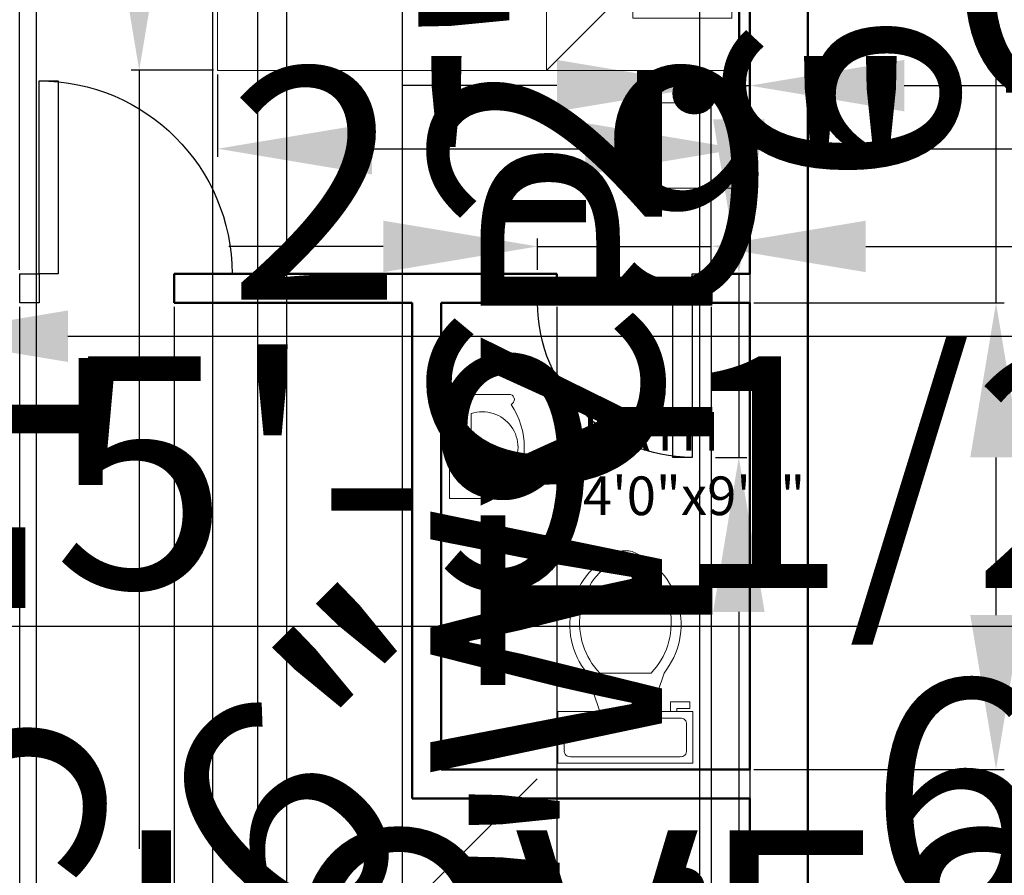
# Model space of a CAD drawing. Units: inches. Extents: x 1102 to 2414, y 295 to 1561.
# Tile 7 of 11: x 1695 to 1848, y 894 to 1027. Entities that reach past the tile are written whole.
import ezdxf

# ---------------------------------------------------------------- set-up
doc = ezdxf.new("R2010")
doc.units = ezdxf.units.IN
for name, color, linetype, lineweight in [('A-ANNO-DIMS', 2, 'Continuous', 18), ('A-AREA-IDEN', 7, 'Continuous', 25), ('A-DOOR', 4, 'Continuous', 25), ('A-FLOR-FIXT', 9, 'Continuous', 18), ('A-FURN', 8, 'Continuous', 18), ('A-WALL', 7, 'Continuous', 50)]:
    doc.layers.add(name, color=color, linetype=linetype, lineweight=lineweight)
doc.styles.get("Standard").update_dxf_attribs({"font": 'arial.ttf'})
doc.dimstyles.new('ISO-25', dxfattribs={"dimtxt": 36, "dimasz": 24, "dimexe": 1.25, "dimexo": 0.625, "dimtad": 1, "dimlunit": 4, "dimtxsty": 'Standard', "dimcen": 2.5, "dimadec": 0, "dimazin": 0, "dimtfac": 1, "dimtmove": 0, "dimatfit": 3, "dimfxl": 1, "dimarcsym": 0})

# ---------------------------------------------------------------- blocks, each defined once
blk = doc.blocks.new('*D3')
at = {"layer": 'A-ANNO-DIMS', "color": 0, "lineweight": -2, "transparency": 16777216}
for p, q in [((1818.17, 1116.76), (1895.42, 1116.76)), ((1894.17, 1092.76), (1894.17, 660.76)), ((1818.17, 636.76), (1895.42, 636.76))]:
    blk.add_line(p, q, dxfattribs=at)
at = {"layer": 'A-ANNO-DIMS', "color": 0, "transparency": 16777216}
for points in [[(1890.17, 1092.76), (1898.17, 1092.76), (1894.17, 1116.76)], [(1890.17, 660.76), (1898.17, 660.76), (1894.17, 636.76)]]:
    blk.add_solid(points, dxfattribs=at)
at = {"layer": 'Defpoints', "color": 0, "transparency": 16777216}
for p in [(1817.54, 1116.76), (1817.54, 636.76), (1894.17, 636.76)]:
    blk.add_point(p, dxfattribs=at)
at = {"layer": 'A-ANNO-DIMS', "color": 0, "transparency": 16777216, "insert": (1875.16, 876.76), "char_height": 36, "attachment_point": 5, "rotation": 90}
blk.add_mtext("40'", dxfattribs=at)
blk = doc.blocks.new('Toilet - top')
for p, q in [((9.5, -6), (9.5, -2)), ((-10, -8.5), (-8, -8.5)), ((-10, -9.5), (-10, -8.5)), ((-8, -8.5), (-8, -8)), ((-7, -8), (-7, -9.5)), ((-4, -8), (-6, -14)), ((4, -8), (6, -14)), ((-7, -9.5), (-10, -9.5)), ((4, -14), (-4, -14))]:
    blk.add_line(p, q)
blk.add_lwpolyline([(10.5, -8), (10.5, 0), (-10.5, 0), (-10.5, -8)], close=True)
for points in [[(8.5, -1), (-8.5, -1)], [(-9.5, -2), (-9.5, -6)], [(-8.5, -7), (8.5, -7)]]:
    blk.add_lwpolyline(points)
for centre, radius, start, end in [((-8.62, -1.88), 0.884, 81.8699, 188.1301), ((8.62, -1.88), 0.884, 351.8699, 98.1301), ((-8.62, -6.12), 0.884, 171.8699, 278.1301), ((8.62, -6.12), 0.884, 261.8699, 8.1301), ((3.52, -21.58), 12.17, 141.4691, 247.9714), ((4.2, -21.82), 11.33, 136.3677, 238.9468), ((-3.52, -21.58), 12.17, 292.0284, 38.5307), ((-4.2, -21.82), 11.33, 301.053, 43.6321), ((0, -27.88), 4, 245.7318, 294.2682), ((0, -29), 4, 254.8605, 285.1395)]:
    blk.add_arc(centre, radius, start, end)
blk = doc.blocks.new('Bed - Queen')
for p, q in [((0, -80.00003), (0, 0)), ((0, 0), (59.99999, 0)), ((59.99999, 0), (59.99999, -80.00003)), ((7.99999, -1.2), (28.79998, -1.2)), ((7.99999, -14.4), (7.99999, -1.2)), ((28.79998, -1.2), (28.79998, -14.4)), ((31.19999, -1.2), (51.99999, -1.2)), ((31.19999, -14.4), (31.19999, -1.2)), ((51.99999, -1.2), (51.99999, -16.4)), ((0, -14.4), (44.8, -14.4)), ((59.99999, -29.6), (44.8, -14.4)), ((44.8, -14.4), (44.8, -29.6)), ((51.99999, -16.4), (46.79936, -16.4)), ((44.8, -16.8), (0, -16.8)), ((44.8, -29.6), (59.99999, -29.6)), ((59.99999, -80.00003), (0, -80.00003))]:
    blk.add_line(p, q)
blk = doc.blocks.new('roomdoor')
for points in [[(1837.54, 1413.02), (1840.54, 1413.02), (1840.54, 1443.02), (1837.54, 1443.02)], [(1840.54, 1408.52), (1843.54, 1408.52), (1843.54, 1413.02), (1840.54, 1413.02)]]:
    blk.add_lwpolyline(points, close=True)
blk.add_arc((1840.54, 1413.02), 30, 90, 180)
blk = doc.blocks.new('utilitydoor')
for points in [[(1891.43, 1413.69), (1894.43, 1413.69), (1894.43, 1437.69), (1891.43, 1437.69)], [(1894.43, 1409.19), (1897.43, 1409.19), (1897.43, 1413.69), (1894.43, 1413.69)]]:
    blk.add_lwpolyline(points, close=True)
blk.add_arc((1894.43, 1413.69), 24, 90, 180)
blk = doc.blocks.new('TABLE-BEDSIDE')
for p, q in [((16.99, 13.29), (0, 13.29)), ((0, 13.29), (0, 0)), ((2.56, 0), (2.56, 13.29)), ((16.99, 0), (16.99, 13.29)), ((0, 0), (16.99, 0))]:
    blk.add_line(p, q)
blk = doc.blocks.new('*D18')
at = {"layer": 'A-ANNO-DIMS', "color": 0, "lineweight": -2, "transparency": 16777216}
for p, q in [((1646.02, 927.81), (1646.02, 951.81)), ((1643.89, 903.81), (1647.27, 903.81)), ((1646.02, 903.81), (1646.02, 894.61)), ((1643.89, 894.6), (1647.27, 894.61)), ((1646.03, 870.61), (1646.05, 625.92))]:
    blk.add_line(p, q, dxfattribs=at)
at = {"layer": 'A-ANNO-DIMS', "color": 0, "transparency": 16777216}
for points in [[(1650.02, 927.81), (1642.02, 927.81), (1646.02, 903.81)], [(1650.03, 870.61), (1642.03, 870.6), (1646.02, 894.61)]]:
    blk.add_solid(points, dxfattribs=at)
at = {"layer": 'Defpoints', "color": 0, "transparency": 16777216}
for p in [(1643.27, 903.81), (1643.27, 894.6), (1646.02, 894.61)]:
    blk.add_point(p, dxfattribs=at)
at = {"layer": 'A-ANNO-DIMS', "color": 0, "transparency": 16777216, "insert": (1665.05, 736.26), "char_height": 36, "attachment_point": 5, "rotation": 270.0057}
blk.add_mtext('0\'-9" TYP.', dxfattribs=at)
blk = doc.blocks.new('*D20')
at = {"layer": 'A-ANNO-DIMS', "color": 0, "lineweight": -2, "transparency": 16777216}
for p, q in [((1808.58, 695.77), (1808.58, 1020.95)), ((1806.65, 671.77), (1809.83, 671.77)), ((1808.58, 658.48), (1808.58, 671.77)), ((1806.65, 658.48), (1809.83, 658.48)), ((1808.58, 634.48), (1808.58, 610.48))]:
    blk.add_line(p, q, dxfattribs=at)
at = {"layer": 'A-ANNO-DIMS', "color": 0, "transparency": 16777216}
for points in [[(1804.58, 695.77), (1812.58, 695.77), (1808.58, 671.77)], [(1804.58, 634.48), (1812.58, 634.48), (1808.58, 658.48)]]:
    blk.add_solid(points, dxfattribs=at)
at = {"layer": 'Defpoints', "color": 0, "transparency": 16777216}
for p in [(1806.03, 671.77), (1808.58, 671.77), (1806.03, 658.48)]:
    blk.add_point(p, dxfattribs=at)
at = {"layer": 'A-ANNO-DIMS', "color": 0, "transparency": 16777216, "insert": (1789.34, 870.36), "char_height": 36, "attachment_point": 5, "rotation": 90}
blk.add_mtext('1\'-1 1/2" TYP.', dxfattribs=at)
blk = doc.blocks.new('*D23')
at = {"layer": 'A-ANNO-DIMS', "color": 0, "lineweight": -2, "transparency": 16777216}
for p, q in [((1725.8, 1018.76), (1725.8, 1005.96)), ((1806.97, 1018.76), (1806.97, 1005.96)), ((1749.8, 1007.21), (1782.97, 1007.21)), ((1806.97, 1007.21), (2238.05, 1007.21))]:
    blk.add_line(p, q, dxfattribs=at)
at = {"layer": 'A-ANNO-DIMS', "color": 0, "transparency": 16777216}
for points in [[(1749.8, 1011.21), (1749.8, 1003.21), (1725.8, 1007.21)], [(1782.97, 1011.21), (1782.97, 1003.21), (1806.97, 1007.21)]]:
    blk.add_solid(points, dxfattribs=at)
at = {"layer": 'Defpoints', "color": 0, "transparency": 16777216}
for p in [(1725.8, 1019.39), (1806.97, 1019.39), (1806.97, 1007.21)]:
    blk.add_point(p, dxfattribs=at)
at = {"layer": 'A-ANNO-DIMS', "color": 0, "transparency": 16777216, "insert": (2034.51, 1027.55), "char_height": 36, "attachment_point": 5}
blk.add_mtext('QUEEN BED 6\'-9"', dxfattribs=at)
blk = doc.blocks.new('*D24')
at = {"layer": 'A-ANNO-DIMS', "color": 0, "lineweight": -2, "transparency": 16777216}
for p, q in [((1725.17, 1080.27), (1712.37, 1080.27)), ((1713.62, 1056.27), (1713.62, 1043.39)), ((1725.17, 1019.39), (1712.37, 1019.39)), ((1713.62, 1019.39), (1713.62, 898.44))]:
    blk.add_line(p, q, dxfattribs=at)
at = {"layer": 'A-ANNO-DIMS', "color": 0, "transparency": 16777216}
for points in [[(1709.62, 1056.27), (1717.62, 1056.27), (1713.62, 1080.27)], [(1709.62, 1043.39), (1717.62, 1043.39), (1713.62, 1019.39)]]:
    blk.add_solid(points, dxfattribs=at)
at = {"layer": 'Defpoints', "color": 0, "transparency": 16777216}
for p in [(1725.8, 1080.27), (1713.62, 1019.39), (1725.8, 1019.39)]:
    blk.add_point(p, dxfattribs=at)
at = {"layer": 'A-ANNO-DIMS', "color": 0, "transparency": 16777216, "insert": (1694.62, 946.91), "char_height": 36, "attachment_point": 5, "rotation": 90}
blk.add_mtext('5\'-1"', dxfattribs=at)
blk = doc.blocks.new('*D25')
at = {"layer": 'A-ANNO-DIMS', "color": 0, "lineweight": -2, "transparency": 16777216}
for p, q in [((1800.76, 877.69), (1800.76, 1221.61)), ((1796.43, 853.69), (1802.01, 853.69)), ((1800.76, 820.65), (1800.76, 853.69)), ((1796.43, 820.65), (1802.01, 820.65)), ((1800.76, 796.65), (1800.76, 772.65))]:
    blk.add_line(p, q, dxfattribs=at)
at = {"layer": 'A-ANNO-DIMS', "color": 0, "transparency": 16777216}
for points in [[(1796.76, 877.69), (1804.76, 877.69), (1800.76, 853.69)], [(1796.76, 796.65), (1804.76, 796.65), (1800.76, 820.65)]]:
    blk.add_solid(points, dxfattribs=at)
at = {"layer": 'Defpoints', "color": 0, "transparency": 16777216}
for p in [(1795.81, 853.69), (1800.76, 853.69), (1795.81, 820.65)]:
    blk.add_point(p, dxfattribs=at)
at = {"layer": 'A-ANNO-DIMS', "color": 0, "transparency": 16777216, "insert": (1781.53, 1061.65), "char_height": 36, "attachment_point": 5, "rotation": 90}
blk.add_mtext('WC 2\'-9" TYP.', dxfattribs=at)
blk = doc.blocks.new('*D27')
at = {"layer": 'A-ANNO-DIMS', "color": 0, "lineweight": -2, "transparency": 16777216}
for p, q in [((1683.72, 1041.76), (1683.72, 1561.36)), ((1679.17, 1017.76), (1684.97, 1017.76)), ((1683.72, 983.26), (1683.72, 1017.76)), ((1679.17, 983.26), (1684.97, 983.26)), ((1683.72, 959.26), (1683.72, 935.26))]:
    blk.add_line(p, q, dxfattribs=at)
at = {"layer": 'A-ANNO-DIMS', "color": 0, "transparency": 16777216}
for points in [[(1679.72, 1041.76), (1687.72, 1041.76), (1683.72, 1017.76)], [(1679.72, 959.26), (1687.72, 959.26), (1683.72, 983.26)]]:
    blk.add_solid(points, dxfattribs=at)
at = {"layer": 'Defpoints', "color": 0, "transparency": 16777216}
for p in [(1678.54, 1017.76), (1683.72, 1017.76), (1678.54, 983.26)]:
    blk.add_point(p, dxfattribs=at)
at = {"layer": 'A-ANNO-DIMS', "color": 0, "transparency": 16777216, "insert": (1664.47, 1313.56), "char_height": 36, "attachment_point": 5, "rotation": 90}
blk.add_mtext('DOOR 2\'-10 1/2" TYP.', dxfattribs=at)
blk = doc.blocks.new('*D28')
at = {"layer": 'A-ANNO-DIMS', "color": 0, "lineweight": -2, "transparency": 16777216}
for p, q in [((1645.54, 982.63), (1645.54, 976.83)), ((1678.54, 982.63), (1678.54, 976.83)), ((1621.54, 978.08), (1597.54, 978.08)), ((1645.54, 978.08), (1678.54, 978.08)), ((1702.54, 978.08), (1947.85, 978.08))]:
    blk.add_line(p, q, dxfattribs=at)
at = {"layer": 'A-ANNO-DIMS', "color": 0, "transparency": 16777216}
for points in [[(1621.54, 982.08), (1621.54, 974.08), (1645.54, 978.08)], [(1702.54, 982.08), (1702.54, 974.08), (1678.54, 978.08)]]:
    blk.add_solid(points, dxfattribs=at)
at = {"layer": 'Defpoints', "color": 0, "transparency": 16777216}
for p in [(1645.54, 983.26), (1678.54, 983.26), (1678.54, 978.08)]:
    blk.add_point(p, dxfattribs=at)
at = {"layer": 'A-ANNO-DIMS', "color": 0, "transparency": 16777216, "insert": (1837.19, 997.09), "char_height": 36, "attachment_point": 5}
blk.add_mtext('2\'-9" TYP.', dxfattribs=at)
blk = doc.blocks.new('*D29')
at = {"layer": 'A-ANNO-DIMS', "color": 0, "lineweight": -2, "transparency": 16777216}
for p, q in [((1806.82, 1011.76), (1806.82, 1035.76)), ((1803.17, 987.76), (1808.07, 987.76)), ((1806.82, 987.76), (1806.82, 959.26)), ((1803.17, 959.26), (1808.07, 959.26)), ((1806.82, 935.26), (1806.82, 295.33))]:
    blk.add_line(p, q, dxfattribs=at)
at = {"layer": 'A-ANNO-DIMS', "color": 0, "transparency": 16777216}
for points in [[(1802.82, 1011.76), (1810.82, 1011.76), (1806.82, 987.76)], [(1802.82, 935.26), (1810.82, 935.26), (1806.82, 959.26)]]:
    blk.add_solid(points, dxfattribs=at)
at = {"layer": 'Defpoints', "color": 0, "transparency": 16777216}
for p in [(1802.54, 987.76), (1802.54, 959.26), (1806.82, 959.26)]:
    blk.add_point(p, dxfattribs=at)
at = {"layer": 'A-ANNO-DIMS', "color": 0, "transparency": 16777216, "insert": (1787.57, 603.3), "char_height": 36, "attachment_point": 5, "rotation": 90}
blk.add_mtext('BATH DOOR 2\'-4 1/2" TYP.', dxfattribs=at)
blk = doc.blocks.new('*D30')
at = {"layer": 'A-ANNO-DIMS', "color": 0, "lineweight": -2, "transparency": 16777216}
for p, q in [((1775.54, 988.38), (1775.54, 993.28)), ((1802.54, 988.38), (1802.54, 993.28)), ((1751.54, 992.03), (1727.54, 992.03)), ((1775.54, 992.03), (1802.54, 992.03)), ((1826.54, 992.03), (2071.85, 992.03))]:
    blk.add_line(p, q, dxfattribs=at)
at = {"layer": 'A-ANNO-DIMS', "color": 0, "transparency": 16777216}
for points in [[(1751.54, 996.03), (1751.54, 988.03), (1775.54, 992.03)], [(1826.54, 996.03), (1826.54, 988.03), (1802.54, 992.03)]]:
    blk.add_solid(points, dxfattribs=at)
at = {"layer": 'Defpoints', "color": 0, "transparency": 16777216}
for p in [(1802.54, 992.03), (1775.54, 987.76), (1802.54, 987.76)]:
    blk.add_point(p, dxfattribs=at)
at = {"layer": 'A-ANNO-DIMS', "color": 0, "transparency": 16777216, "insert": (1961.19, 1011.05), "char_height": 36, "attachment_point": 5}
blk.add_mtext('2\'-3" TYP.', dxfattribs=at)
blk = doc.blocks.new('*D31')
at = {"layer": 'A-ANNO-DIMS', "color": 0, "lineweight": -2, "transparency": 16777216}
for p, q in [((1629.86, 764.63), (1629.86, 760.41)), ((1653.86, 764.63), (1653.86, 760.41)), ((1605.86, 761.66), (1581.86, 761.66)), ((1629.86, 761.66), (1653.86, 761.66)), ((1677.86, 761.66), (2225.36, 761.66))]:
    blk.add_line(p, q, dxfattribs=at)
at = {"layer": 'A-ANNO-DIMS', "color": 0, "transparency": 16777216}
for points in [[(1605.86, 765.66), (1605.86, 757.66), (1629.86, 761.66)], [(1677.86, 765.66), (1677.86, 757.66), (1653.86, 761.66)]]:
    blk.add_solid(points, dxfattribs=at)
at = {"layer": 'Defpoints', "color": 0, "transparency": 16777216}
for p in [(1629.86, 765.26), (1653.86, 765.26), (1653.86, 761.66)]:
    blk.add_point(p, dxfattribs=at)
at = {"layer": 'A-ANNO-DIMS', "color": 0, "transparency": 16777216, "insert": (1963.61, 780.91), "char_height": 36, "attachment_point": 5}
blk.add_mtext('DOOR LEAF 2\'-0" TYP.', dxfattribs=at)
blk = doc.blocks.new('*D32')
at = {"layer": 'A-ANNO-DIMS', "color": 0, "lineweight": -2, "transparency": 16777216}
for p, q in [((1657.46, 811.76), (1657.46, 1164.91)), ((1654.49, 787.76), (1658.71, 787.76)), ((1657.46, 765.26), (1657.46, 787.76)), ((1654.49, 765.26), (1658.71, 765.26)), ((1657.46, 741.26), (1657.46, 717.26))]:
    blk.add_line(p, q, dxfattribs=at)
at = {"layer": 'A-ANNO-DIMS', "color": 0, "transparency": 16777216}
for points in [[(1653.46, 811.76), (1661.46, 811.76), (1657.46, 787.76)], [(1653.46, 741.26), (1661.46, 741.26), (1657.46, 765.26)]]:
    blk.add_solid(points, dxfattribs=at)
at = {"layer": 'Defpoints', "color": 0, "transparency": 16777216}
for p in [(1653.86, 787.76), (1657.46, 787.76), (1653.86, 765.26)]:
    blk.add_point(p, dxfattribs=at)
at = {"layer": 'A-ANNO-DIMS', "color": 0, "transparency": 16777216, "insert": (1638.22, 1000.34), "char_height": 36, "attachment_point": 5, "rotation": 90}
blk.add_mtext('1\'-10 1/2" TYP.', dxfattribs=at)
blk = doc.blocks.new('*D39')
at = {"layer": 'A-ANNO-DIMS', "color": 0, "lineweight": -2, "transparency": 16777216}
for p, q in [((1623.32, 855.67), (1623.32, 860.64)), ((1652.27, 855.67), (1652.27, 860.64)), ((1599.32, 859.39), (1575.32, 859.39)), ((1623.32, 859.39), (1652.27, 859.39)), ((1676.27, 859.39), (2075.12, 859.39))]:
    blk.add_line(p, q, dxfattribs=at)
at = {"layer": 'A-ANNO-DIMS', "color": 0, "transparency": 16777216}
for points in [[(1599.32, 863.39), (1599.32, 855.39), (1623.32, 859.39)], [(1676.27, 863.39), (1676.27, 855.39), (1652.27, 859.39)]]:
    blk.add_solid(points, dxfattribs=at)
at = {"layer": 'Defpoints', "color": 0, "transparency": 16777216}
for p in [(1652.27, 859.39), (1623.32, 855.05), (1652.27, 855.05)]:
    blk.add_point(p, dxfattribs=at)
at = {"layer": 'A-ANNO-DIMS', "color": 0, "transparency": 16777216, "insert": (1887.69, 878.64), "char_height": 36, "attachment_point": 5}
blk.add_mtext('LOVESEAT 2\'-5"', dxfattribs=at)
blk = doc.blocks.new('*D45')
at = {"layer": 'A-ANNO-DIMS', "color": 0, "lineweight": -2, "transparency": 16777216}
for p, q in [((1736.54, 770.38), (1736.54, 1147.26)), ((1754.54, 770.38), (1754.54, 1147.26)), ((1712.54, 1146.01), (1688.54, 1146.01)), ((1736.54, 1146.01), (1754.54, 1146.01)), ((1778.54, 1146.01), (1896.1, 1146.01))]:
    blk.add_line(p, q, dxfattribs=at)
at = {"layer": 'A-ANNO-DIMS', "color": 0, "transparency": 16777216}
for points in [[(1712.54, 1150.01), (1712.54, 1142.01), (1736.54, 1146.01)], [(1778.54, 1150.01), (1778.54, 1142.01), (1754.54, 1146.01)]]:
    blk.add_solid(points, dxfattribs=at)
at = {"layer": 'Defpoints', "color": 0, "transparency": 16777216}
for p in [(1754.54, 1146.01), (1736.54, 769.76), (1754.54, 769.76)]:
    blk.add_point(p, dxfattribs=at)
at = {"layer": 'A-ANNO-DIMS', "color": 0, "transparency": 16777216, "insert": (1849.32, 1165.02), "char_height": 36, "attachment_point": 5}
blk.add_mtext('1\'-6"', dxfattribs=at)
blk = doc.blocks.new('*D47')
at = {"layer": 'A-ANNO-DIMS', "color": 0, "lineweight": -2, "transparency": 16777216}
for p, q in [((1736.54, 854.38), (1736.54, 884.26)), ((1808.54, 854.38), (1808.54, 884.26)), ((1760.54, 883.01), (1784.54, 883.01)), ((1808.54, 883.01), (1929.69, 883.01))]:
    blk.add_line(p, q, dxfattribs=at)
at = {"layer": 'A-ANNO-DIMS', "color": 0, "transparency": 16777216}
for points in [[(1760.54, 887.01), (1760.54, 879.01), (1736.54, 883.01)], [(1784.54, 887.01), (1784.54, 879.01), (1808.54, 883.01)]]:
    blk.add_solid(points, dxfattribs=at)
at = {"layer": 'Defpoints', "color": 0, "transparency": 16777216}
for p in [(1808.54, 883.01), (1736.54, 853.76), (1808.54, 853.76)]:
    blk.add_point(p, dxfattribs=at)
at = {"layer": 'A-ANNO-DIMS', "color": 0, "transparency": 16777216, "insert": (1881.12, 902.02), "char_height": 36, "attachment_point": 5}
blk.add_mtext('6\'-0"', dxfattribs=at)
blk = doc.blocks.new('*D48')
at = {"layer": 'A-ANNO-DIMS', "color": 0, "lineweight": -2, "transparency": 16777216}
for p, q in [((1689.04, 854.38), (1689.04, 1147.26)), ((1732.04, 858.88), (1732.04, 1147.26)), ((1665.04, 1146.01), (1641.04, 1146.01)), ((1689.04, 1146.01), (1732.04, 1146.01)), ((1756.04, 1146.01), (1876.97, 1146.01))]:
    blk.add_line(p, q, dxfattribs=at)
at = {"layer": 'A-ANNO-DIMS', "color": 0, "transparency": 16777216}
for points in [[(1665.04, 1150.01), (1665.04, 1142.01), (1689.04, 1146.01)], [(1756.04, 1150.01), (1756.04, 1142.01), (1732.04, 1146.01)]]:
    blk.add_solid(points, dxfattribs=at)
at = {"layer": 'Defpoints', "color": 0, "transparency": 16777216}
for p in [(1732.04, 1146.01), (1732.04, 858.26), (1689.04, 853.76)]:
    blk.add_point(p, dxfattribs=at)
at = {"layer": 'A-ANNO-DIMS', "color": 0, "transparency": 16777216, "insert": (1828.51, 1165.03), "char_height": 36, "attachment_point": 5}
blk.add_mtext('3\'-7"', dxfattribs=at)
blk = doc.blocks.new('*D49')
at = {"layer": 'A-ANNO-DIMS', "color": 0, "lineweight": -2, "transparency": 16777216}
for p, q in [((1846.79, 983.26), (1846.79, 1188.29)), ((1809.17, 983.26), (1848.04, 983.26)), ((1846.79, 934.76), (1846.79, 959.26)), ((1809.17, 910.76), (1848.04, 910.76))]:
    blk.add_line(p, q, dxfattribs=at)
at = {"layer": 'A-ANNO-DIMS', "color": 0, "transparency": 16777216}
for points in [[(1842.79, 959.26), (1850.79, 959.26), (1846.79, 983.26)], [(1842.79, 934.76), (1850.79, 934.76), (1846.79, 910.76)]]:
    blk.add_solid(points, dxfattribs=at)
at = {"layer": 'Defpoints', "color": 0, "transparency": 16777216}
for p in [(1808.54, 983.26), (1846.79, 983.26), (1808.54, 910.76)]:
    blk.add_point(p, dxfattribs=at)
at = {"layer": 'A-ANNO-DIMS', "color": 0, "transparency": 16777216, "insert": (1827.56, 1097.77), "char_height": 36, "attachment_point": 5, "rotation": 90}
blk.add_mtext('6\'-0 1/2"', dxfattribs=at)
blk = doc.blocks.new('*D50')
at = {"layer": 'A-ANNO-DIMS', "color": 0, "lineweight": -2, "transparency": 16777216}
for p, q in [((1586.54, 987.13), (1586.54, 606.26)), ((1654.54, 987.13), (1654.54, 606.26)), ((1610.54, 607.51), (1630.54, 607.51)), ((1654.54, 607.51), (1775.49, 607.51))]:
    blk.add_line(p, q, dxfattribs=at)
at = {"layer": 'A-ANNO-DIMS', "color": 0, "transparency": 16777216}
for points in [[(1610.54, 611.51), (1610.54, 603.51), (1586.54, 607.51)], [(1630.54, 611.51), (1630.54, 603.51), (1654.54, 607.51)]]:
    blk.add_solid(points, dxfattribs=at)
at = {"layer": 'Defpoints', "color": 0, "transparency": 16777216}
for p in [(1586.54, 987.76), (1654.54, 987.76), (1654.54, 607.51)]:
    blk.add_point(p, dxfattribs=at)
at = {"layer": 'A-ANNO-DIMS', "color": 0, "transparency": 16777216, "insert": (1727.02, 626.52), "char_height": 36, "attachment_point": 5}
blk.add_mtext('5\'-8"', dxfattribs=at)
blk = doc.blocks.new('*D51')
at = {"layer": 'A-ANNO-DIMS', "color": 0, "lineweight": -2, "transparency": 16777216}
for p, q in [((1689.04, 988.38), (1689.04, 1147.26)), ((1695.04, 988.38), (1695.04, 1147.26)), ((1665.04, 1146.01), (1641.04, 1146.01)), ((1689.04, 1146.01), (1695.04, 1146.01)), ((1719.04, 1146.01), (1839.99, 1146.01))]:
    blk.add_line(p, q, dxfattribs=at)
at = {"layer": 'A-ANNO-DIMS', "color": 0, "transparency": 16777216}
for points in [[(1665.04, 1150.01), (1665.04, 1142.01), (1689.04, 1146.01)], [(1719.04, 1150.01), (1719.04, 1142.01), (1695.04, 1146.01)]]:
    blk.add_solid(points, dxfattribs=at)
at = {"layer": 'Defpoints', "color": 0, "transparency": 16777216}
for p in [(1695.04, 1146.01), (1689.04, 987.76), (1695.04, 987.76)]:
    blk.add_point(p, dxfattribs=at)
at = {"layer": 'A-ANNO-DIMS', "color": 0, "transparency": 16777216, "insert": (1791.52, 1165.02), "char_height": 36, "attachment_point": 5}
blk.add_mtext('0\'-6"', dxfattribs=at)
blk = doc.blocks.new('*D52')
at = {"layer": 'A-ANNO-DIMS', "color": 0, "lineweight": -2, "transparency": 16777216}
for p, q in [((1802.54, 988.38), (1802.54, 1018.26)), ((1808.54, 988.38), (1808.54, 1018.26)), ((1778.54, 1017.01), (1754.54, 1017.01)), ((1802.54, 1017.01), (1808.54, 1017.01)), ((1832.54, 1017.01), (1953.49, 1017.01))]:
    blk.add_line(p, q, dxfattribs=at)
at = {"layer": 'A-ANNO-DIMS', "color": 0, "transparency": 16777216}
for points in [[(1778.54, 1021.01), (1778.54, 1013.01), (1802.54, 1017.01)], [(1832.54, 1021.01), (1832.54, 1013.01), (1808.54, 1017.01)]]:
    blk.add_solid(points, dxfattribs=at)
at = {"layer": 'Defpoints', "color": 0, "transparency": 16777216}
for p in [(1808.54, 1017.01), (1802.54, 987.76), (1808.54, 987.76)]:
    blk.add_point(p, dxfattribs=at)
at = {"layer": 'A-ANNO-DIMS', "color": 0, "transparency": 16777216, "insert": (1905.02, 1036.02), "char_height": 36, "attachment_point": 5}
blk.add_mtext('0\'-6"', dxfattribs=at)
blk = doc.blocks.new('*D53')
at = {"layer": 'A-ANNO-DIMS', "color": 0, "lineweight": -2, "transparency": 16777216}
for p, q in [((1586.54, 988.38), (1586.54, 1147.26)), ((1610.54, 988.38), (1610.54, 1147.26)), ((1562.54, 1146.01), (1538.54, 1146.01)), ((1586.54, 1146.01), (1610.54, 1146.01)), ((1634.54, 1146.01), (1756.11, 1146.01))]:
    blk.add_line(p, q, dxfattribs=at)
at = {"layer": 'A-ANNO-DIMS', "color": 0, "transparency": 16777216}
for points in [[(1562.54, 1150.01), (1562.54, 1142.01), (1586.54, 1146.01)], [(1634.54, 1150.01), (1634.54, 1142.01), (1610.54, 1146.01)]]:
    blk.add_solid(points, dxfattribs=at)
at = {"layer": 'Defpoints', "color": 0, "transparency": 16777216}
for p in [(1610.54, 1146.01), (1586.54, 987.76), (1610.54, 987.76)]:
    blk.add_point(p, dxfattribs=at)
at = {"layer": 'A-ANNO-DIMS', "color": 0, "transparency": 16777216, "insert": (1707.32, 1165.02), "char_height": 36, "attachment_point": 5}
blk.add_mtext('2\'-0"', dxfattribs=at)
blk = doc.blocks.new('*D55')
at = {"layer": 'A-ANNO-DIMS', "color": 0, "lineweight": -2, "transparency": 16777216}
for p, q in [((1586.54, 722.38), (1586.54, 1147.26)), ((1622.54, 722.38), (1622.54, 1147.26)), ((1562.54, 1146.01), (1538.54, 1146.01)), ((1586.54, 1146.01), (1622.54, 1146.01)), ((1646.54, 1146.01), (1767.47, 1146.01))]:
    blk.add_line(p, q, dxfattribs=at)
at = {"layer": 'A-ANNO-DIMS', "color": 0, "transparency": 16777216}
for points in [[(1562.54, 1150.01), (1562.54, 1142.01), (1586.54, 1146.01)], [(1646.54, 1150.01), (1646.54, 1142.01), (1622.54, 1146.01)]]:
    blk.add_solid(points, dxfattribs=at)
at = {"layer": 'Defpoints', "color": 0, "transparency": 16777216}
for p in [(1622.54, 1146.01), (1586.54, 721.76), (1622.54, 721.76)]:
    blk.add_point(p, dxfattribs=at)
at = {"layer": 'A-ANNO-DIMS', "color": 0, "transparency": 16777216, "insert": (1719.01, 1165.03), "char_height": 36, "attachment_point": 5}
blk.add_mtext('3\'-0"', dxfattribs=at)
blk = doc.blocks.new('*D58')
at = {"layer": 'A-ANNO-DIMS', "color": 0, "lineweight": -2, "transparency": 16777216}
for p, q in [((1612.78, 904.43), (1612.78, 934.3)), ((1682.5, 904.43), (1682.5, 934.3)), ((1636.78, 933.05), (1658.5, 933.05)), ((1682.5, 933.05), (1887.33, 933.05))]:
    blk.add_line(p, q, dxfattribs=at)
at = {"layer": 'A-ANNO-DIMS', "color": 0, "transparency": 16777216}
for points in [[(1636.78, 937.05), (1636.78, 929.05), (1612.78, 933.05)], [(1658.5, 937.05), (1658.5, 929.05), (1682.5, 933.05)]]:
    blk.add_solid(points, dxfattribs=at)
at = {"layer": 'Defpoints', "color": 0, "transparency": 16777216}
for p in [(1682.5, 933.05), (1612.78, 903.8), (1682.5, 903.8)]:
    blk.add_point(p, dxfattribs=at)
at = {"layer": 'A-ANNO-DIMS', "color": 0, "transparency": 16777216, "insert": (1796.92, 952.29), "char_height": 36, "attachment_point": 5}
blk.add_mtext('5\'-9 1/2"', dxfattribs=at)
blk = doc.blocks.new('*D62')
at = {"layer": 'A-ANNO-DIMS', "color": 0, "lineweight": -2, "transparency": 16777216}
for p, q in [((1778.54, 982.63), (1778.54, 606.26)), ((1802.54, 982.63), (1802.54, 606.26)), ((1754.54, 607.51), (1730.54, 607.51)), ((1778.54, 607.51), (1802.54, 607.51)), ((1826.54, 607.51), (1948.11, 607.51))]:
    blk.add_line(p, q, dxfattribs=at)
at = {"layer": 'A-ANNO-DIMS', "color": 0, "transparency": 16777216}
for points in [[(1754.54, 611.51), (1754.54, 603.51), (1778.54, 607.51)], [(1826.54, 611.51), (1826.54, 603.51), (1802.54, 607.51)]]:
    blk.add_solid(points, dxfattribs=at)
at = {"layer": 'Defpoints', "color": 0, "transparency": 16777216}
for p in [(1778.54, 983.26), (1802.54, 983.26), (1802.54, 607.51)]:
    blk.add_point(p, dxfattribs=at)
at = {"layer": 'A-ANNO-DIMS', "color": 0, "transparency": 16777216, "insert": (1899.32, 626.52), "char_height": 36, "attachment_point": 5}
blk.add_mtext('2\'-0"', dxfattribs=at)
blk = doc.blocks.new('*D63')
at = {"layer": 'A-ANNO-DIMS', "color": 0, "lineweight": -2, "transparency": 16777216}
for p, q in [((1654.54, 982.63), (1654.54, 606.26)), ((1678.54, 982.63), (1678.54, 606.26)), ((1630.54, 607.51), (1606.54, 607.51)), ((1654.54, 607.51), (1678.54, 607.51)), ((1702.54, 607.51), (1824.11, 607.51))]:
    blk.add_line(p, q, dxfattribs=at)
at = {"layer": 'A-ANNO-DIMS', "color": 0, "transparency": 16777216}
for points in [[(1630.54, 611.51), (1630.54, 603.51), (1654.54, 607.51)], [(1702.54, 611.51), (1702.54, 603.51), (1678.54, 607.51)]]:
    blk.add_solid(points, dxfattribs=at)
at = {"layer": 'Defpoints', "color": 0, "transparency": 16777216}
for p in [(1654.54, 983.26), (1678.54, 983.26), (1678.54, 607.51)]:
    blk.add_point(p, dxfattribs=at)
at = {"layer": 'A-ANNO-DIMS', "color": 0, "transparency": 16777216, "insert": (1775.32, 626.52), "char_height": 36, "attachment_point": 5}
blk.add_mtext('2\'-0"', dxfattribs=at)
blk = doc.blocks.new('*D64')
at = {"layer": 'A-ANNO-DIMS', "color": 0, "lineweight": -2, "transparency": 16777216}
for p, q in [((1695.04, 982.63), (1695.04, 606.26)), ((1719.04, 982.63), (1719.04, 606.26)), ((1671.04, 607.51), (1647.04, 607.51)), ((1695.04, 607.51), (1719.04, 607.51)), ((1743.04, 607.51), (1864.61, 607.51))]:
    blk.add_line(p, q, dxfattribs=at)
at = {"layer": 'A-ANNO-DIMS', "color": 0, "transparency": 16777216}
for points in [[(1671.04, 611.51), (1671.04, 603.51), (1695.04, 607.51)], [(1743.04, 611.51), (1743.04, 603.51), (1719.04, 607.51)]]:
    blk.add_solid(points, dxfattribs=at)
at = {"layer": 'Defpoints', "color": 0, "transparency": 16777216}
for p in [(1695.04, 983.26), (1719.04, 983.26), (1719.04, 607.51)]:
    blk.add_point(p, dxfattribs=at)
at = {"layer": 'A-ANNO-DIMS', "color": 0, "transparency": 16777216, "insert": (1815.82, 626.52), "char_height": 36, "attachment_point": 5}
blk.add_mtext('2\'-0"', dxfattribs=at)
blk = doc.blocks.new('*D65')
at = {"layer": 'A-ANNO-DIMS', "color": 0, "lineweight": -2, "transparency": 16777216}
for p, q in [((1697.64, 770.38), (1697.64, 1147.26)), ((1725.04, 770.38), (1725.04, 1147.26)), ((1673.64, 1146.01), (1649.64, 1146.01)), ((1697.64, 1146.01), (1725.04, 1146.01)), ((1749.04, 1146.01), (1954.49, 1146.01))]:
    blk.add_line(p, q, dxfattribs=at)
at = {"layer": 'A-ANNO-DIMS', "color": 0, "transparency": 16777216}
for points in [[(1673.64, 1150.01), (1673.64, 1142.01), (1697.64, 1146.01)], [(1749.04, 1150.01), (1749.04, 1142.01), (1725.04, 1146.01)]]:
    blk.add_solid(points, dxfattribs=at)
at = {"layer": 'Defpoints', "color": 0, "transparency": 16777216}
for p in [(1725.04, 1146.01), (1697.64, 769.76), (1725.04, 769.76)]:
    blk.add_point(p, dxfattribs=at)
at = {"layer": 'A-ANNO-DIMS', "color": 0, "transparency": 16777216, "insert": (1863.77, 1165.26), "char_height": 36, "attachment_point": 5}
blk.add_mtext('2\'-3 1/2"', dxfattribs=at)
blk = doc.blocks.new('*D69')
at = {"layer": 'A-ANNO-DIMS', "color": 0, "lineweight": -2, "transparency": 16777216}
for p, q in [((1775.45, 909.34), (1665.56, 799.46)), ((1635.86, 769.76), (1648.59, 782.49))]:
    blk.add_line(p, q, dxfattribs=at)
at = {"layer": 'A-ANNO-DIMS', "color": 0, "transparency": 16777216}
blk.add_solid([(1662.73, 802.29), (1668.39, 796.63), (1648.59, 782.49)], dxfattribs=at)
at = {"layer": 'Defpoints', "color": 0, "transparency": 16777216}
for p in [(1648.59, 782.49), (1635.86, 769.76)]:
    blk.add_point(p, dxfattribs=at)
at = {"layer": 'A-ANNO-DIMS', "color": 0, "transparency": 16777216, "insert": (1715.55, 876.32), "char_height": 36, "attachment_point": 5, "rotation": 45}
blk.add_mtext('R1\'-6"', dxfattribs=at)

msp = doc.modelspace()

# ---------------------------------------------------------------- linework, layer by layer
at = {"layer": 'A-FLOR-FIXT'}
for p, q in [((1761.831, 969.045), (1761.831, 952.875)), ((1761.831, 969.045), (1771.337, 969.045)), ((1765.204, 966.058), (1765.204, 955.556)), ((1761.831, 952.875), (1771.79, 952.875))]:
    msp.add_line(p, q, dxfattribs=at)
for centre, radius in [((1764.418, 962.549), 0.278), ((1764.716, 960.961), 0.357), ((1766.179, 960.956), 0.451), ((1764.22, 959.453), 0.317)]:
    msp.add_circle(centre, radius, dxfattribs=at)
for centre, radius, start, end in [((1771.089, 968.243), 0.839, 295.5147, 72.79987), ((1761.423, 960.826), 12.037, 326.40939, 33.59061), ((1766.96, 960.807), 5.537, 251.51851, 108.48149), ((1771.224, 953.417), 0.784, 316.25991, 73.17544)]:
    msp.add_arc(centre, radius, start, end, dxfattribs=at)
at = {"layer": 'A-WALL'}
for p, q in [((1817.544, 636.76), (1817.544, 1116.76)), ((1808.544, 987.76), (1808.544, 1107.76)), ((1719.044, 987.76), (1719.044, 983.26)), ((1778.544, 987.76), (1719.044, 987.76)), ((1778.544, 983.26), (1778.544, 987.76)), ((1808.544, 987.76), (1802.544, 987.76)), ((1802.544, 983.26), (1802.544, 987.76)), ((1744.044, 983.26), (1719.044, 983.26)), ((1756.044, 983.26), (1744.044, 983.26)), ((1756.044, 906.26), (1756.044, 983.26)), ((1760.544, 910.76), (1760.544, 983.26)), ((1778.544, 983.26), (1760.544, 983.26)), ((1808.544, 983.26), (1802.544, 983.26)), ((1808.544, 983.26), (1802.544, 983.26)), ((1808.544, 910.76), (1808.544, 983.26)), ((1808.544, 910.76), (1760.544, 910.76)), ((1808.544, 906.26), (1756.044, 906.26)), ((1808.544, 858.26), (1808.544, 906.26))]:
    msp.add_line(p, q, dxfattribs=at)

# ---------------------------------------------------------------- block references
at = {"layer": 'A-DOOR', "xscale": -1}
msp.add_blockref('roomdoor', (3538.588, -425.258), dxfattribs=at)
at = {"layer": 'A-DOOR', "xscale": -1, "rotation": 180}
msp.add_blockref('utilitydoor', (-94.887, 2396.947), dxfattribs=at)
at = {"layer": 'A-FLOR-FIXT', "rotation": 180}
msp.add_blockref('Toilet - top', (1789.191, 911.755), dxfattribs=at)
at = {"layer": 'A-FURN', "xscale": 1.014688796722326, "yscale": 1.014688796722326, "zscale": 1.014688796722326, "rotation": 270}
msp.add_blockref('Bed - Queen', (1806.973, 1080.268), dxfattribs=at)
at = {"layer": 'A-FURN'}
msp.add_blockref('TABLE-BEDSIDE', (1789.09, 1001.072), dxfattribs=at)

# ---------------------------------------------------------------- texts
at = {"layer": 'A-AREA-IDEN', "insert": (1782.573, 966.289), "char_height": 6, "attachment_point": 1}
msp.add_mtext_dynamic_manual_height_columns('BATH\\P4\'0"x9\'0"', width=50.64919, gutter_width=12.5, heights=[0], dxfattribs=at)

# ---------------------------------------------------------------- dimensions: what is measured, and where the dimension line sits
at = {"layer": 'A-ANNO-DIMS'}
for base, p1, p2, angle, text, picture, middle in [((1683.719, 1017.76), (1678.544, 983.26), (1678.544, 1017.76), 90, 'DOOR <> TYP.', '*D27', (1664.468, 1313.559)), ((1800.764, 853.692), (1795.807, 820.646), (1795.807, 853.692), 90, 'WC <> TYP.', '*D25', (1781.525, 1061.653)), ((1657.464, 787.76), (1653.864, 765.26), (1653.864, 787.76), 90, '<> TYP.', '*D32', (1638.225, 1000.337)), ((1806.819, 959.26), (1802.544, 987.76), (1802.544, 959.26), 270, 'BATH DOOR <> TYP.', '*D29', (1787.568, 603.296)), ((1808.577, 671.77), (1806.028, 658.482), (1806.028, 671.77), 90, '<> TYP.', '*D20', (1789.338, 870.362)), ((1646.024, 894.605), (1643.268, 903.806), (1643.269, 894.605), 270.00567, '<> TYP.', '*D18', (1665.045, 736.263))]:
    dim = msp.add_linear_dim(base=base, p1=p1, p2=p2, angle=angle, text=text, dimstyle='ISO-25', override={"dimdec": 1, "dimlfac": 1, "dimrnd": 0, "dimzin": 1, "dimdsep": 46, "dimlunit": 4, "dimfrac": 2}, dxfattribs=at)
    dim.commit()
    dim.dimension.update_dxf_attribs({"geometry": picture, "text_midpoint": middle})
for base, p1, p2, picture, middle in [((1725.044, 1146.01), (1697.644, 769.76), (1725.044, 769.76), '*D65', (1863.767, 1165.261)), ((1622.544, 1146.01), (1586.544, 721.76), (1622.544, 721.76), '*D55', (1719.005, 1165.028)), ((1610.544, 1146.01), (1586.544, 987.76), (1610.544, 987.76), '*D53', (1707.325, 1165.015)), ((1732.044, 1146.01), (1689.044, 853.76), (1732.044, 858.26), '*D48', (1828.505, 1165.028)), ((1695.044, 1146.01), (1689.044, 987.76), (1695.044, 987.76), '*D51', (1791.518, 1165.015)), ((1754.544, 1146.01), (1736.544, 769.76), (1754.544, 769.76), '*D45', (1849.323, 1165.015)), ((1808.544, 1017.01), (1802.544, 987.76), (1808.544, 987.76), '*D52', (1905.018, 1036.015)), ((1682.499, 933.053), (1612.778, 903.803), (1682.499, 903.803), '*D58', (1796.915, 952.292)), ((1654.544, 607.51), (1586.544, 987.76), (1654.544, 987.76), '*D50', (1727.018, 626.515)), ((1678.544, 607.51), (1654.544, 983.26), (1678.544, 983.26), '*D63', (1775.325, 626.515)), ((1719.044, 607.51), (1695.044, 983.26), (1719.044, 983.26), '*D64', (1815.825, 626.515)), ((1802.544, 607.51), (1778.544, 983.26), (1802.544, 983.26), '*D62', (1899.325, 626.515)), ((1808.544, 883.01), (1736.544, 853.76), (1808.544, 853.76), '*D47', (1881.116, 902.015))]:
    dim = msp.add_linear_dim(base=base, p1=p1, p2=p2, dimstyle='ISO-25', override={"dimdec": 1, "dimlfac": 1, "dimrnd": 0, "dimzin": 1, "dimdsep": 46, "dimlunit": 4, "dimfrac": 2}, dxfattribs=at)
    dim.commit()
    dim.dimension.update_dxf_attribs({"geometry": picture, "text_midpoint": middle})
for base, p1, p2, angle, picture, middle in [((1846.794, 983.26), (1808.544, 910.76), (1808.544, 983.26), 90, '*D49', (1827.555, 1097.774)), ((1713.621, 1019.387), (1725.798, 1080.268), (1725.798, 1019.387), 270, '*D24', (1694.616, 946.913))]:
    dim = msp.add_linear_dim(base=base, p1=p1, p2=p2, angle=angle, dimstyle='ISO-25', override={"dimdec": 1, "dimlfac": 1, "dimrnd": 0, "dimzin": 1, "dimdsep": 46, "dimlunit": 4, "dimfrac": 2}, dxfattribs=at)
    dim.commit()
    dim.dimension.update_dxf_attribs({"geometry": picture, "text_midpoint": middle})
dim = msp.add_linear_dim(base=(1894.167, 636.76), p1=(1817.544, 1116.76), p2=(1817.544, 636.76), angle=90, dimstyle='ISO-25', override={"dimclrd": 0, "dimclre": 0, "dimclrt": 0}, dxfattribs=at)
dim.commit()
dim.dimension.update_dxf_attribs({"geometry": '*D3', "text_midpoint": (1894.167, 876.76), "dimtype": 160})
for base, p1, p2, text, picture, middle in [((1806.973, 1007.211), (1725.798, 1019.387), (1806.973, 1019.387), 'QUEEN BED <>', '*D23', (2034.509, 1027.555)), ((1802.544, 992.035), (1775.544, 987.76), (1802.544, 987.76), '<> TYP.', '*D30', (1961.195, 1011.053)), ((1678.544, 978.085), (1645.544, 983.26), (1678.544, 983.26), '<> TYP.', '*D28', (1837.195, 997.09)), ((1652.268, 859.388), (1623.32, 855.046), (1652.268, 855.046), 'LOVESEAT <>', '*D39', (1887.695, 878.64)), ((1653.864, 761.66), (1629.864, 765.26), (1653.864, 765.26), 'DOOR LEAF <> TYP.', '*D31', (1963.611, 780.911))]:
    dim = msp.add_linear_dim(base=base, p1=p1, p2=p2, text=text, dimstyle='ISO-25', override={"dimdec": 1, "dimlfac": 1, "dimrnd": 0, "dimzin": 1, "dimdsep": 46, "dimlunit": 4, "dimfrac": 2}, dxfattribs=at)
    dim.commit()
    dim.dimension.update_dxf_attribs({"geometry": picture, "text_midpoint": middle})
dim = msp.add_radius_dim(center=(1635.864, 769.76), mpoint=(1648.592, 782.488), dimstyle='ISO-25', override={"dimdec": 1, "dimlfac": 1, "dimrnd": 0, "dimzin": 1, "dimdsep": 46, "dimlunit": 4, "dimfrac": 2}, dxfattribs=at)
dim.commit()
dim.dimension.update_dxf_attribs({"geometry": '*D69', "text_midpoint": (1715.551, 876.325)})

doc.saveas('drawing.dxf')
